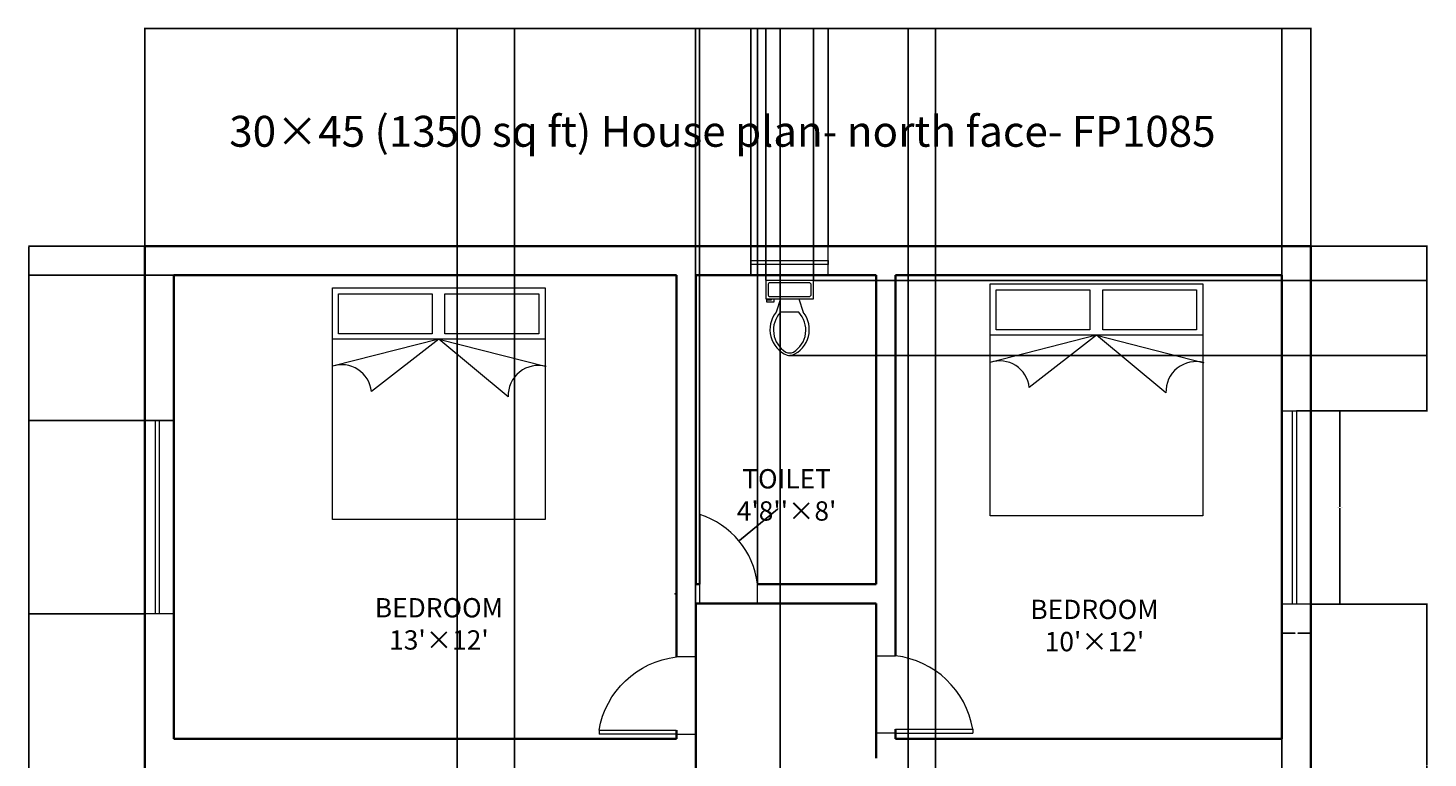
# Model space of a CAD drawing. Units: inches. Extents: x 1108 to 1543, y 442 to 1097.
# Tile 3 of 3: x 1108 to 1543, y 871 to 1097. Entities that reach past the tile are written whole.
import ezdxf

# ---------------------------------------------------------------- set-up
doc = ezdxf.new("R2010")
doc.units = ezdxf.units.IN
for name, color, linetype, lineweight in [('A-ANNO-DIMS', 2, 'Continuous', 18), ('A-ANNO-TEXT', 7, 'Continuous', 25), ('A-AREA-IDEN', 7, 'Continuous', 18), ('A-DOOR', 4, 'Continuous', 18), ('A-FLOR-FIXT', 9, 'Continuous', 18), ('A-FURN', 8, 'Continuous', 18), ('A-GLAZ', 5, 'Continuous', 18), ('A-WALL', 7, 'Continuous', 35)]:
    doc.layers.add(name, color=color, linetype=linetype, lineweight=lineweight)
doc.styles.get("Standard").update_dxf_attribs({"font": 'times.ttf'})
doc.dimstyles.get("Standard").update_dxf_attribs({"dimtxt": 0.18, "dimasz": 0.18, "dimexe": 0.18, "dimexo": 0.0625, "dimgap": 0.09, "dimtad": 0, "dimtih": 1, "dimtoh": 1, "dimdec": 4, "dimzin": 0, "dimdsep": 46, "dimtxsty": 'Standard', "dimcen": 0.09, "dimadec": 0, "dimazin": 0, "dimtfac": 1, "dimtdec": 4, "dimtofl": 0, "dimtmove": 0, "dimatfit": 3, "dimfxl": 1, "dimtolj": 1, "dimtzin": 0, "dimarcsym": 0})

# ---------------------------------------------------------------- blocks, each defined once
blk = doc.blocks.new('d')
for p, q in [((1309.33, 626.48), (1285.33, 626.48)), ((1285.33, 625.28), (1285.33, 626.48)), ((1309.33, 626.48), (1315.33, 626.48)), ((1309.33, 625.28), (1285.33, 625.28)), ((1315.33, 602.48), (1309.33, 602.48))]:
    blk.add_line(p, q)
blk.add_arc((1312.52, 629.86), 27.57, 189.5705, 263.3671)
blk = doc.blocks.new('*U3')
for p, q in [((9.5, -6), (9.5, -2)), ((-10, -8.5), (-8, -8.5)), ((-10, -9.5), (-10, -8.5)), ((-7, -9.5), (-10, -9.5)), ((-8, -8.5), (-8, -8)), ((-7, -8), (-7, -9.5)), ((-4, -8), (-6, -14)), ((4, -8), (6, -14)), ((4, -14), (-4, -14))]:
    blk.add_line(p, q)
blk.add_lwpolyline([(10.5, -8), (10.5, 0), (-10.5, 0), (-10.5, -8)], close=True)
for points in [[(-9.5, -2), (-9.5, -6)], [(8.5, -1), (-8.5, -1)], [(-8.5, -7), (8.5, -7)]]:
    blk.add_lwpolyline(points)
for centre, radius, start, end in [((-8.62, -1.88), 0.884, 81.8699, 188.1301), ((-8.62, -6.12), 0.884, 171.8699, 278.1301), ((8.62, -1.88), 0.884, 351.8699, 98.1301), ((8.62, -6.12), 0.884, 261.8699, 8.1301), ((3.52, -21.58), 12.17, 141.46911, 247.97143), ((4.2, -21.82), 11.33, 136.36773, 238.94682), ((-3.52, -21.58), 12.17, 292.02843, 38.53071), ((-4.2, -21.82), 11.33, 301.05301, 43.63209), ((0, -27.88), 4, 245.73182, 294.26817), ((0, -29), 4, 254.86053, 285.13947)]:
    blk.add_arc(centre, radius, start, end)
blk = doc.blocks.new('BED-DOUBLE-66X72')
for p, q in [((0, 0), (0, 72)), ((0, 72), (66, 72)), ((66, 72), (66, 0)), ((66, 56.1), (0, 56.1)), ((33, 56.1), (0, 47.62)), ((33, 56.1), (12.08, 39.84)), ((33, 56.1), (66, 47.62)), ((54.54, 38.14), (33, 56.1)), ((66, 0), (0, 0))]:
    blk.add_line(p, q)
for points in [[(30.92, 70.13), (30.92, 57.75), (1.83, 57.75), (1.83, 70.13)], [(64.01, 70.13), (64.01, 57.75), (34.92, 57.75), (34.92, 70.13)]]:
    blk.add_lwpolyline(points, close=True)
for centre, radius, start, end in [((2.92, 38.89), 9.21, 5.9499, 108.4921), ((63.85, 38.55), 9.32, 74.4856, 182.5542)]:
    blk.add_arc(centre, radius, start, end)
blk = doc.blocks.new('WIN-60IN')
for p, q in [((-9, -60), (-9, 0)), ((-9, 0), (0, 0)), ((-5.7, -60), (-5.7, 0)), ((0, 0), (-4.5, 0)), ((-4.5, 0), (-4.5, -60)), ((0, 0), (0, -60)), ((0, -60), (-9, -60)), ((-4.5, -60), (-5.7, -60))]:
    blk.add_line(p, q)
blk = doc.blocks.new('*D7')
at = {"layer": 'A-ANNO-DIMS', "color": 0, "lineweight": -2, "transparency": 16777216}
for p, q in [((1506.4, 978.47), (1515.51, 978.47)), ((1515.33, 978.29), (1515.33, 948.65)), ((1515.33, 918.65), (1515.33, 948.29)), ((1506.4, 918.47), (1515.51, 918.47))]:
    blk.add_line(p, q, dxfattribs=at)
at = {"layer": 'A-ANNO-DIMS', "color": 0, "transparency": 16777216}
for points in [[(1515.3, 978.29), (1515.36, 978.29), (1515.33, 978.47)], [(1515.3, 918.65), (1515.36, 918.65), (1515.33, 918.47)]]:
    blk.add_solid(points, dxfattribs=at)
at = {"layer": 'Defpoints', "color": 0, "transparency": 16777216}
for p in [(1506.33, 978.47), (1515.33, 978.47), (1506.33, 918.47)]:
    blk.add_point(p, dxfattribs=at)
at = {"layer": 'A-ANNO-DIMS', "color": 0, "transparency": 16777216, "insert": (1515.33, 948.47), "char_height": 0.18, "attachment_point": 5}
blk.add_mtext('\\A1;WINDOW 60 TYP.', dxfattribs=at)
blk = doc.blocks.new('*D8')
at = {"layer": 'A-ANNO-DIMS', "color": 0, "lineweight": -2, "transparency": 16777216}
for p, q in [((1497.33, 918.41), (1497.33, 909.29)), ((1506.33, 918.41), (1506.33, 909.29)), ((1497.51, 909.47), (1501.38, 909.47)), ((1506.15, 909.47), (1502.29, 909.47))]:
    blk.add_line(p, q, dxfattribs=at)
at = {"layer": 'A-ANNO-DIMS', "color": 0, "transparency": 16777216}
for points in [[(1497.51, 909.5), (1497.51, 909.44), (1497.33, 909.47)], [(1506.15, 909.5), (1506.15, 909.44), (1506.33, 909.47)]]:
    blk.add_solid(points, dxfattribs=at)
at = {"layer": 'Defpoints', "color": 0, "transparency": 16777216}
for p in [(1497.33, 918.47), (1506.33, 918.47), (1506.33, 909.47)]:
    blk.add_point(p, dxfattribs=at)
at = {"layer": 'A-ANNO-DIMS', "color": 0, "transparency": 16777216, "insert": (1501.83, 909.47), "char_height": 0.18, "attachment_point": 5}
blk.add_mtext('\\A1;9 TYP.', dxfattribs=at)
blk = doc.blocks.new('*D15')
at = {"layer": 'A-ANNO-DIMS', "color": 0, "lineweight": -2, "transparency": 16777216}
for p, q in [((1144.33, 1029.74), (1144.33, 1097.43)), ((1144.51, 1097.25), (1325.06, 1097.25)), ((1506.15, 1097.25), (1325.61, 1097.25)), ((1506.33, 1029.74), (1506.33, 1097.43))]:
    blk.add_line(p, q, dxfattribs=at)
at = {"layer": 'A-ANNO-DIMS', "color": 0, "transparency": 16777216}
for points in [[(1144.51, 1097.28), (1144.51, 1097.22), (1144.33, 1097.25)], [(1506.15, 1097.28), (1506.15, 1097.22), (1506.33, 1097.25)]]:
    blk.add_solid(points, dxfattribs=at)
at = {"layer": 'Defpoints', "color": 0, "transparency": 16777216}
for p in [(1506.33, 1097.25), (1144.33, 1029.68), (1506.33, 1029.68)]:
    blk.add_point(p, dxfattribs=at)
at = {"layer": 'A-ANNO-DIMS', "color": 0, "transparency": 16777216, "insert": (1325.33, 1097.25), "char_height": 0.18, "attachment_point": 5}
blk.add_mtext('\\A1;362', dxfattribs=at)
blk = doc.blocks.new('*D16')
at = {"layer": 'A-ANNO-DIMS', "color": 0, "lineweight": -2, "transparency": 16777216}
for p, q in [((1144.27, 1029.68), (1108.2, 1029.68)), ((1108.38, 1029.5), (1108.38, 758.36)), ((1108.38, 486.86), (1108.38, 758)), ((1144.27, 486.68), (1108.2, 486.68))]:
    blk.add_line(p, q, dxfattribs=at)
at = {"layer": 'A-ANNO-DIMS', "color": 0, "transparency": 16777216}
for points in [[(1108.35, 1029.5), (1108.41, 1029.5), (1108.38, 1029.68)], [(1108.35, 486.86), (1108.41, 486.86), (1108.38, 486.68)]]:
    blk.add_solid(points, dxfattribs=at)
at = {"layer": 'Defpoints', "color": 0, "transparency": 16777216}
for p in [(1108.38, 1029.68), (1144.33, 1029.68), (1144.33, 486.68)]:
    blk.add_point(p, dxfattribs=at)
at = {"layer": 'A-ANNO-DIMS', "color": 0, "transparency": 16777216, "insert": (1108.38, 758.18), "char_height": 0.18, "attachment_point": 5}
blk.add_mtext('\\A1;543', dxfattribs=at)
blk = doc.blocks.new('*D17')
at = {"layer": 'A-ANNO-DIMS', "color": 0, "lineweight": -2, "transparency": 16777216}
for p, q in [((1153.27, 1020.68), (1108.2, 1020.68)), ((1108.38, 1020.5), (1108.38, 998.26)), ((1108.38, 975.66), (1108.38, 997.9)), ((1153.27, 975.48), (1108.2, 975.48))]:
    blk.add_line(p, q, dxfattribs=at)
at = {"layer": 'A-ANNO-DIMS', "color": 0, "transparency": 16777216}
for points in [[(1108.35, 1020.5), (1108.41, 1020.5), (1108.38, 1020.68)], [(1108.35, 975.66), (1108.41, 975.66), (1108.38, 975.48)]]:
    blk.add_solid(points, dxfattribs=at)
at = {"layer": 'Defpoints', "color": 0, "transparency": 16777216}
for p in [(1153.33, 1020.68), (1108.38, 975.48), (1153.33, 975.48)]:
    blk.add_point(p, dxfattribs=at)
at = {"layer": 'A-ANNO-DIMS', "color": 0, "transparency": 16777216, "insert": (1108.38, 998.08), "char_height": 0.18, "attachment_point": 5}
blk.add_mtext('\\A1;45.2', dxfattribs=at)
blk = doc.blocks.new('*D18')
at = {"layer": 'A-ANNO-DIMS', "color": 0, "lineweight": -2, "transparency": 16777216}
for p, q in [((1144.27, 915.48), (1108.2, 915.48)), ((1108.38, 915.3), (1108.38, 883.28)), ((1108.38, 850.9), (1108.38, 882.92)), ((1144.27, 850.72), (1108.2, 850.72))]:
    blk.add_line(p, q, dxfattribs=at)
at = {"layer": 'A-ANNO-DIMS', "color": 0, "transparency": 16777216}
for points in [[(1108.35, 915.3), (1108.41, 915.3), (1108.38, 915.48)], [(1108.35, 850.9), (1108.41, 850.9), (1108.38, 850.72)]]:
    blk.add_solid(points, dxfattribs=at)
at = {"layer": 'Defpoints', "color": 0, "transparency": 16777216}
for p in [(1144.33, 915.48), (1108.38, 850.72), (1144.33, 850.72)]:
    blk.add_point(p, dxfattribs=at)
at = {"layer": 'A-ANNO-DIMS', "color": 0, "transparency": 16777216, "insert": (1108.38, 883.1), "char_height": 0.18, "attachment_point": 5}
blk.add_mtext('\\A1;64.76', dxfattribs=at)
blk = doc.blocks.new('*D20')
at = {"layer": 'A-ANNO-DIMS', "color": 0, "lineweight": -2, "transparency": 16777216}
for p, q in [((1506.4, 1029.68), (1542.46, 1029.68)), ((1542.28, 1029.5), (1542.28, 1004.26)), ((1542.28, 978.65), (1542.28, 1003.89)), ((1506.4, 978.47), (1542.46, 978.47))]:
    blk.add_line(p, q, dxfattribs=at)
at = {"layer": 'A-ANNO-DIMS', "color": 0, "transparency": 16777216}
for points in [[(1542.25, 1029.5), (1542.31, 1029.5), (1542.28, 1029.68)], [(1542.25, 978.65), (1542.31, 978.65), (1542.28, 978.47)]]:
    blk.add_solid(points, dxfattribs=at)
at = {"layer": 'Defpoints', "color": 0, "transparency": 16777216}
for p in [(1506.33, 1029.68), (1506.33, 978.47), (1542.28, 978.47)]:
    blk.add_point(p, dxfattribs=at)
at = {"layer": 'A-ANNO-DIMS', "color": 0, "transparency": 16777216, "insert": (1542.28, 1004.08), "char_height": 0.18, "attachment_point": 5}
blk.add_mtext('\\A1;51.21', dxfattribs=at)
blk = doc.blocks.new('*D21')
at = {"layer": 'A-ANNO-DIMS', "color": 0, "lineweight": -2, "transparency": 16777216}
for p, q in [((1506.4, 918.47), (1542.46, 918.47)), ((1542.28, 918.29), (1542.28, 868.51)), ((1542.28, 818.36), (1542.28, 868.14)), ((1506.4, 818.18), (1542.46, 818.18))]:
    blk.add_line(p, q, dxfattribs=at)
at = {"layer": 'A-ANNO-DIMS', "color": 0, "transparency": 16777216}
for points in [[(1542.25, 918.29), (1542.31, 918.29), (1542.28, 918.47)], [(1542.25, 818.36), (1542.31, 818.36), (1542.28, 818.18)]]:
    blk.add_solid(points, dxfattribs=at)
at = {"layer": 'Defpoints', "color": 0, "transparency": 16777216}
for p in [(1506.33, 918.47), (1506.33, 818.18), (1542.28, 818.18)]:
    blk.add_point(p, dxfattribs=at)
at = {"layer": 'A-ANNO-DIMS', "color": 0, "transparency": 16777216, "insert": (1542.28, 868.33), "char_height": 0.18, "attachment_point": 5}
blk.add_mtext('\\A1;100.3', dxfattribs=at)
blk = doc.blocks.new('*D26')
at = {"layer": 'A-ANNO-DIMS', "color": 0, "lineweight": -2, "transparency": 16777216}
for p, q in [((1341.52, 495.74), (1341.52, 1097.43)), ((1341.7, 1097.25), (1361.06, 1097.25)), ((1381.15, 1097.25), (1361.8, 1097.25)), ((1381.33, 495.74), (1381.33, 1097.43))]:
    blk.add_line(p, q, dxfattribs=at)
at = {"layer": 'A-ANNO-DIMS', "color": 0, "transparency": 16777216}
for points in [[(1341.7, 1097.28), (1341.7, 1097.22), (1341.52, 1097.25)], [(1381.15, 1097.28), (1381.15, 1097.22), (1381.33, 1097.25)]]:
    blk.add_solid(points, dxfattribs=at)
at = {"layer": 'Defpoints', "color": 0, "transparency": 16777216}
for p in [(1381.33, 1097.25), (1341.52, 495.68), (1381.33, 495.68)]:
    blk.add_point(p, dxfattribs=at)
at = {"layer": 'A-ANNO-DIMS', "color": 0, "transparency": 16777216, "insert": (1361.43, 1097.25), "char_height": 0.18, "attachment_point": 5}
blk.add_mtext('\\A1;39.81', dxfattribs=at)
blk = doc.blocks.new('*D27')
at = {"layer": 'A-ANNO-DIMS', "color": 0, "lineweight": -2, "transparency": 16777216}
for p, q in [((1332.5, 1029.74), (1332.5, 1097.43)), ((1332.68, 1097.25), (1344.29, 1097.25)), ((1356.32, 1097.25), (1344.72, 1097.25)), ((1356.5, 1029.74), (1356.5, 1097.43))]:
    blk.add_line(p, q, dxfattribs=at)
at = {"layer": 'A-ANNO-DIMS', "color": 0, "transparency": 16777216}
for points in [[(1332.68, 1097.28), (1332.68, 1097.22), (1332.5, 1097.25)], [(1356.32, 1097.28), (1356.32, 1097.22), (1356.5, 1097.25)]]:
    blk.add_solid(points, dxfattribs=at)
at = {"layer": 'Defpoints', "color": 0, "transparency": 16777216}
for p in [(1356.5, 1097.25), (1332.5, 1029.68), (1356.5, 1029.68)]:
    blk.add_point(p, dxfattribs=at)
at = {"layer": 'A-ANNO-DIMS', "color": 0, "transparency": 16777216, "insert": (1344.5, 1097.25), "char_height": 0.18, "attachment_point": 5}
blk.add_mtext('\\A1;24', dxfattribs=at)
blk = doc.blocks.new('*D28')
at = {"layer": 'A-ANNO-DIMS', "color": 0, "lineweight": -2, "transparency": 16777216}
for p, q in [((1315.33, 1020.74), (1315.33, 1097.43)), ((1315.51, 1097.25), (1323.48, 1097.25)), ((1332.32, 1097.25), (1324.35, 1097.25)), ((1332.5, 1020.74), (1332.5, 1097.43))]:
    blk.add_line(p, q, dxfattribs=at)
at = {"layer": 'A-ANNO-DIMS', "color": 0, "transparency": 16777216}
for points in [[(1315.51, 1097.28), (1315.51, 1097.22), (1315.33, 1097.25)], [(1332.32, 1097.28), (1332.32, 1097.22), (1332.5, 1097.25)]]:
    blk.add_solid(points, dxfattribs=at)
at = {"layer": 'Defpoints', "color": 0, "transparency": 16777216}
for p in [(1332.5, 1097.25), (1315.33, 1020.68), (1332.5, 1020.68)]:
    blk.add_point(p, dxfattribs=at)
at = {"layer": 'A-ANNO-DIMS', "color": 0, "transparency": 16777216, "insert": (1323.92, 1097.25), "char_height": 0.18, "attachment_point": 5}
blk.add_mtext('\\A1;17.166', dxfattribs=at)
blk = doc.blocks.new('*D29')
at = {"layer": 'A-ANNO-DIMS', "color": 0, "lineweight": -2, "transparency": 16777216}
for p, q in [((1337.1, 1019.05), (1337.1, 1097.43)), ((1337.28, 1097.25), (1344.15, 1097.25)), ((1351.73, 1097.25), (1344.86, 1097.25)), ((1351.91, 1019.05), (1351.91, 1097.43))]:
    blk.add_line(p, q, dxfattribs=at)
at = {"layer": 'A-ANNO-DIMS', "color": 0, "transparency": 16777216}
for points in [[(1337.28, 1097.28), (1337.28, 1097.22), (1337.1, 1097.25)], [(1351.73, 1097.28), (1351.73, 1097.22), (1351.91, 1097.25)]]:
    blk.add_solid(points, dxfattribs=at)
at = {"layer": 'Defpoints', "color": 0, "transparency": 16777216}
for p in [(1351.91, 1097.25), (1337.1, 1018.98), (1351.91, 1018.98)]:
    blk.add_point(p, dxfattribs=at)
at = {"layer": 'A-ANNO-DIMS', "color": 0, "transparency": 16777216, "insert": (1344.5, 1097.25), "char_height": 0.18, "attachment_point": 5}
blk.add_mtext('\\A1;14.81', dxfattribs=at)
blk = doc.blocks.new('*D30')
at = {"layer": 'A-ANNO-DIMS', "color": 0, "lineweight": -2, "transparency": 16777216}
for p, q in [((1351.97, 1018.98), (1542.46, 1018.98)), ((1542.28, 1018.8), (1542.28, 1007.53)), ((1542.28, 995.89), (1542.28, 1007.17)), ((1344.56, 995.71), (1542.46, 995.71))]:
    blk.add_line(p, q, dxfattribs=at)
at = {"layer": 'A-ANNO-DIMS', "color": 0, "transparency": 16777216}
for points in [[(1542.25, 1018.8), (1542.31, 1018.8), (1542.28, 1018.98)], [(1542.25, 995.89), (1542.31, 995.89), (1542.28, 995.71)]]:
    blk.add_solid(points, dxfattribs=at)
at = {"layer": 'Defpoints', "color": 0, "transparency": 16777216}
for p in [(1351.91, 1018.98), (1542.28, 1018.98), (1344.5, 995.71)]:
    blk.add_point(p, dxfattribs=at)
at = {"layer": 'A-ANNO-DIMS', "color": 0, "transparency": 16777216, "insert": (1542.28, 1007.35), "char_height": 0.18, "attachment_point": 5}
blk.add_mtext('\\A1;23.273', dxfattribs=at)
blk = doc.blocks.new('*D31')
at = {"layer": 'A-ANNO-DIMS', "color": 0, "lineweight": -2, "transparency": 16777216}
for p, q in [((1316.53, 946.34), (1316.53, 1097.43)), ((1316.71, 1097.25), (1325.33, 1097.25)), ((1334.35, 1097.25), (1325.73, 1097.25)), ((1334.53, 924.74), (1334.53, 1097.43))]:
    blk.add_line(p, q, dxfattribs=at)
at = {"layer": 'A-ANNO-DIMS', "color": 0, "transparency": 16777216}
for points in [[(1316.71, 1097.28), (1316.71, 1097.22), (1316.53, 1097.25)], [(1334.35, 1097.28), (1334.35, 1097.22), (1334.53, 1097.25)]]:
    blk.add_solid(points, dxfattribs=at)
at = {"layer": 'Defpoints', "color": 0, "transparency": 16777216}
for p in [(1334.53, 1097.25), (1316.53, 946.28), (1334.53, 924.68)]:
    blk.add_point(p, dxfattribs=at)
at = {"layer": 'A-ANNO-DIMS', "color": 0, "transparency": 16777216, "insert": (1325.53, 1097.25), "char_height": 0.18, "attachment_point": 5}
blk.add_mtext('\\A1;18', dxfattribs=at)
blk = doc.blocks.new('*D49')
at = {"layer": 'A-ANNO-DIMS', "color": 0, "lineweight": -2, "transparency": 16777216}
for p, q in [((1241.29, 854.74), (1241.29, 1097.43)), ((1241.47, 1097.25), (1249.81, 1097.25)), ((1258.89, 1097.25), (1250.55, 1097.25)), ((1259.07, 854.74), (1259.07, 1097.43))]:
    blk.add_line(p, q, dxfattribs=at)
at = {"layer": 'A-ANNO-DIMS', "color": 0, "transparency": 16777216}
for points in [[(1241.47, 1097.28), (1241.47, 1097.22), (1241.29, 1097.25)], [(1258.89, 1097.28), (1258.89, 1097.22), (1259.07, 1097.25)]]:
    blk.add_solid(points, dxfattribs=at)
at = {"layer": 'Defpoints', "color": 0, "transparency": 16777216}
for p in [(1259.07, 1097.25), (1241.29, 854.68), (1259.07, 854.68)]:
    blk.add_point(p, dxfattribs=at)
at = {"layer": 'A-ANNO-DIMS', "color": 0, "transparency": 16777216, "insert": (1250.18, 1097.25), "char_height": 0.18, "attachment_point": 5}
blk.add_mtext('\\A1;17.78', dxfattribs=at)
blk = doc.blocks.new('*D50')
at = {"layer": 'A-ANNO-DIMS', "color": 0, "lineweight": -2, "transparency": 16777216}
for p, q in [((1381.33, 537.14), (1381.33, 1097.43)), ((1381.51, 1097.25), (1385.16, 1097.25)), ((1389.56, 1097.25), (1385.91, 1097.25)), ((1389.74, 537.14), (1389.74, 1097.43))]:
    blk.add_line(p, q, dxfattribs=at)
at = {"layer": 'A-ANNO-DIMS', "color": 0, "transparency": 16777216}
for points in [[(1381.51, 1097.28), (1381.51, 1097.22), (1381.33, 1097.25)], [(1389.56, 1097.28), (1389.56, 1097.22), (1389.74, 1097.25)]]:
    blk.add_solid(points, dxfattribs=at)
at = {"layer": 'Defpoints', "color": 0, "transparency": 16777216}
for p in [(1389.74, 1097.25), (1381.33, 537.08), (1389.74, 537.08)]:
    blk.add_point(p, dxfattribs=at)
at = {"layer": 'A-ANNO-DIMS', "color": 0, "transparency": 16777216, "insert": (1385.54, 1097.25), "char_height": 0.18, "attachment_point": 5}
blk.add_mtext('\\A1;8.404', dxfattribs=at)
blk = doc.blocks.new('*D52')
at = {"layer": 'A-ANNO-DIMS', "color": 0, "lineweight": -2, "transparency": 16777216}
for p, q in [((1315.33, 573.74), (1315.33, 1097.43)), ((1315.51, 1097.25), (1406.07, 1097.25)), ((1497.15, 1097.25), (1406.6, 1097.25)), ((1497.33, 573.74), (1497.33, 1097.43))]:
    blk.add_line(p, q, dxfattribs=at)
at = {"layer": 'A-ANNO-DIMS', "color": 0, "transparency": 16777216}
for points in [[(1315.51, 1097.28), (1315.51, 1097.22), (1315.33, 1097.25)], [(1497.15, 1097.28), (1497.15, 1097.22), (1497.33, 1097.25)]]:
    blk.add_solid(points, dxfattribs=at)
at = {"layer": 'Defpoints', "color": 0, "transparency": 16777216}
for p in [(1497.33, 1097.25), (1315.33, 573.68), (1497.33, 573.68)]:
    blk.add_point(p, dxfattribs=at)
at = {"layer": 'A-ANNO-DIMS', "color": 0, "transparency": 16777216, "insert": (1406.33, 1097.25), "char_height": 0.18, "attachment_point": 5}
blk.add_mtext('\\A1;182', dxfattribs=at)
blk = doc.blocks.new('*D53')
at = {"layer": 'A-ANNO-DIMS', "color": 0, "lineweight": -2, "transparency": 16777216}
for p, q in [((1340.69, 948), (1328.92, 938.24)), ((1340.87, 948), (1340.69, 948)), ((1308.84, 921.68), (1309.02, 921.68)), ((1308.93, 921.59), (1308.93, 921.77))]:
    blk.add_line(p, q, dxfattribs=at)
at = {"layer": 'A-ANNO-DIMS', "color": 0, "transparency": 16777216}
blk.add_solid([(1328.9, 938.27), (1328.94, 938.22), (1328.78, 938.13)], dxfattribs=at)
at = {"layer": 'Defpoints', "color": 0, "transparency": 16777216}
for p in [(1328.78, 938.13), (1308.93, 921.68)]:
    blk.add_point(p, dxfattribs=at)
at = {"layer": 'A-ANNO-DIMS', "color": 0, "transparency": 16777216, "insert": (1341.34, 948), "char_height": 0.18, "attachment_point": 5}
blk.add_mtext('\\A1;R25.78', dxfattribs=at)

msp = doc.modelspace()

# ---------------------------------------------------------------- linework, layer by layer
at = {"layer": 'A-DOOR'}
for p, q in [((1316.5347, 924.6791), (1316.5347, 946.2791)), ((1316.5347, 946.2791), (1316.6347, 946.2791)), ((1316.6347, 946.2791), (1316.6347, 924.6791)), ((1316.6347, 924.6791), (1315.3347, 924.6791)), ((1316.5347, 924.6791), (1316.5347, 918.6791)), ((1316.5347, 924.6791), (1316.6347, 924.6791)), ((1334.5347, 918.6791), (1334.5347, 924.6791)), ((1316.5347, 918.6791), (1334.5347, 918.6791))]:
    msp.add_line(p, q, dxfattribs=at)
msp.add_arc((1308.9321, 921.6791), 25.7777, 6.683214, 72.614123, dxfattribs=at)
at = {"layer": 'A-GLAZ'}
for p, q in [((1356.5008, 1029.6791), (1332.5008, 1029.6791)), ((1332.5008, 1029.6791), (1332.5008, 1020.6791)), ((1356.5008, 1020.6791), (1356.5008, 1029.6791)), ((1332.5008, 1025.1791), (1356.5008, 1025.1791)), ((1356.5008, 1023.9791), (1332.5008, 1023.9791)), ((1356.5008, 1025.1791), (1356.5008, 1023.9791)), ((1332.5008, 1020.6791), (1356.5008, 1020.6791))]:
    msp.add_line(p, q, dxfattribs=at)
at = {"layer": 'A-WALL'}
for p, q in [((1144.3347, 486.6791), (1144.3347, 1029.6791)), ((1144.3347, 1029.6791), (1506.3347, 1029.6791)), ((1506.3347, 486.6791), (1506.3347, 1029.6791)), ((1153.3347, 876.6791), (1153.3347, 1020.6791)), ((1153.3347, 1020.6791), (1309.3347, 1020.6791)), ((1309.3347, 1020.6791), (1309.3347, 902.0778)), ((1315.3347, 1020.6791), (1315.3347, 924.6791)), ((1315.3347, 1020.6791), (1315.3347, 924.6791)), ((1315.3347, 1020.6791), (1371.3347, 1020.6791)), ((1371.3347, 1020.6791), (1371.3347, 924.6791)), ((1377.3347, 1020.6791), (1377.3347, 924.6791)), ((1377.3347, 1020.6791), (1497.3347, 1020.6791)), ((1497.3347, 876.6791), (1497.3347, 1020.6791)), ((1315.3347, 924.6791), (1316.5347, 924.6791)), ((1371.3347, 924.6791), (1334.5347, 924.6791)), ((1377.3347, 918.6791), (1377.3347, 924.6791)), ((1315.3347, 918.6791), (1371.3347, 918.6791)), ((1315.3347, 918.6791), (1315.3347, 828.2882)), ((1371.3347, 918.6791), (1371.3347, 870.6791)), ((1377.3347, 918.6791), (1377.3347, 902.4167)), ((1309.3347, 879.2778), (1309.3347, 876.6791)), ((1377.3347, 879.6167), (1377.3347, 876.6791)), ((1153.3347, 876.6791), (1309.3347, 876.6791)), ((1377.3347, 876.6791), (1497.3347, 876.6791))]:
    msp.add_line(p, q, dxfattribs=at)

# ---------------------------------------------------------------- block references
at = {"layer": 'A-DOOR', "xscale": -1, "rotation": 180}
msp.add_blockref('d', (0, 1504.5569), dxfattribs=at)
at = {"layer": 'A-DOOR', "rotation": 180}
msp.add_blockref('d', (2686.6693, 1504.8958), dxfattribs=at)
at = {"layer": 'A-FLOR-FIXT', "xscale": 0.7052287925630897, "yscale": 0.7052287925630897, "zscale": 0.7052287925630897}
msp.add_blockref('*U3', (1344.5024, 1018.9841), dxfattribs=at)
at = {"layer": 'A-FURN'}
for p in [(1406.7886, 945.9341), (1202.5883, 944.7248)]:
    msp.add_blockref('BED-DOUBLE-66X72', p, dxfattribs=at)
at = {"layer": 'A-GLAZ'}
for p in [(1506.3347, 978.4725), (1153.3347, 975.4836)]:
    msp.add_blockref('WIN-60IN', p, dxfattribs=at)

# ---------------------------------------------------------------- texts
at = {"layer": 'A-ANNO-TEXT', "insert": (1132.9515, 1070.1369), "char_height": 9.6, "attachment_point": 1}
msp.add_mtext_dynamic_manual_height_columns('\\pxqc;30×45 (1350 sq ft) House plan- north face- FP1085', width=381.364536, gutter_width=12.5, heights=[0], dxfattribs=at)
at = {"layer": 'A-AREA-IDEN', "char_height": 6, "attachment_point": 1}
for s, insert in [("\\pxqc;TOILET\\P4'8''×8'", (1209.0015, 960.4092)), ("\\pxqc;BEDROOM \\P13'×12'", (1101.0866, 920.3526)), ("\\pxqc;BEDROOM \\P10'×12'", (1304.5832, 919.839))]:
    msp.add_mtext_dynamic_manual_height_columns(s, width=269.09847, gutter_width=12.5, heights=[0], dxfattribs=dict(at, insert=insert))

# ---------------------------------------------------------------- dimensions: what is measured, and where the dimension line sits
at = {"layer": 'A-ANNO-DIMS'}
for base, p1, p2, override, picture, middle in [((1506.3347, 1097.2479), (1144.3347, 1029.6791), (1506.3347, 1029.6791), {"dimdec": 0, "dimlfac": 1, "dimrnd": 0, "dimzin": 0, "dimdsep": 46, "dimlunit": 2}, '*D15', (1325.3347, 1097.2479)), ((1259.07, 1097.2479), (1241.2895, 854.6808), (1259.07, 854.6808), {"dimdec": 2, "dimlfac": 1, "dimrnd": 0, "dimzin": 0, "dimdsep": 46, "dimlunit": 2}, '*D49', (1250.1797, 1097.2479)), ((1332.5008, 1097.2479), (1315.3347, 1020.6791), (1332.5008, 1020.6791), {"dimdec": 3, "dimlfac": 1, "dimrnd": 0, "dimzin": 0, "dimdsep": 46, "dimlunit": 2}, '*D28', (1323.9177, 1097.2479)), ((1497.3347, 1097.2479), (1315.3347, 573.6791), (1497.3347, 573.6791), {"dimdec": 0, "dimlfac": 1, "dimrnd": 0, "dimzin": 0, "dimdsep": 46, "dimlunit": 2}, '*D52', (1406.3347, 1097.2479)), ((1334.5347, 1097.2479), (1316.5347, 946.2791), (1334.5347, 924.6791), {"dimdec": 0, "dimlfac": 1, "dimrnd": 0, "dimzin": 0, "dimdsep": 46, "dimlunit": 2}, '*D31', (1325.5347, 1097.2479)), ((1356.5008, 1097.2479), (1332.5008, 1029.6791), (1356.5008, 1029.6791), {"dimdec": 0, "dimlfac": 1, "dimrnd": 0, "dimzin": 0, "dimdsep": 46, "dimlunit": 2}, '*D27', (1344.5008, 1097.2479)), ((1351.9073, 1097.2479), (1337.0975, 1018.9841), (1351.9073, 1018.9841), {"dimdec": 2, "dimlfac": 1, "dimrnd": 0, "dimzin": 0, "dimdsep": 46, "dimlunit": 2}, '*D29', (1344.5024, 1097.2479)), ((1381.3347, 1097.2479), (1341.5247, 495.6791), (1381.3347, 495.6791), {"dimdec": 2, "dimlfac": 1, "dimrnd": 0, "dimzin": 0, "dimdsep": 46, "dimlunit": 2}, '*D26', (1361.4297, 1097.2479)), ((1389.7386, 1097.2479), (1381.3347, 537.0791), (1389.7386, 537.0791), {"dimdec": 3, "dimlfac": 1, "dimrnd": 0, "dimzin": 0, "dimdsep": 46, "dimlunit": 2}, '*D50', (1385.5366, 1097.2479))]:
    dim = msp.add_linear_dim(base=base, p1=p1, p2=p2, dimstyle='Standard', override=override, dxfattribs=at)
    dim.commit()
    dim.dimension.update_dxf_attribs({"geometry": picture, "text_midpoint": middle})
for base, p1, p2, override, picture, middle in [((1108.3847, 1029.6791), (1144.3347, 486.6791), (1144.3347, 1029.6791), {"dimdec": 0, "dimlfac": 1, "dimrnd": 0, "dimzin": 0, "dimdsep": 46, "dimlunit": 2}, '*D16', (1108.3847, 758.1791)), ((1542.2847, 978.4725), (1506.3347, 1029.6791), (1506.3347, 978.4725), {"dimdec": 2, "dimlfac": 1, "dimrnd": 0, "dimzin": 0, "dimdsep": 46, "dimlunit": 2}, '*D20', (1542.2847, 1004.0758)), ((1108.3847, 975.4836), (1153.3347, 1020.6791), (1153.3347, 975.4836), {"dimdec": 1, "dimlfac": 1, "dimrnd": 0, "dimzin": 0, "dimdsep": 46, "dimlunit": 2}, '*D17', (1108.3847, 998.0813)), ((1542.28466, 1018.98414), (1344.50239, 995.71161), (1351.90728, 1018.98414), {"dimdec": 3, "dimlfac": 1, "dimrnd": 0, "dimzin": 0, "dimdsep": 46, "dimlunit": 2}, '*D30', (1542.28466, 1007.34787)), ((1542.2847, 818.1791), (1506.3347, 918.4725), (1506.3347, 818.1791), {"dimdec": 1, "dimlfac": 1, "dimrnd": 0, "dimzin": 0, "dimdsep": 46, "dimlunit": 2}, '*D21', (1542.2847, 868.3258)), ((1108.3847, 850.719), (1144.3347, 915.4836), (1144.3347, 850.719), {"dimdec": 2, "dimlfac": 1, "dimrnd": 0, "dimzin": 0, "dimdsep": 46, "dimlunit": 2}, '*D18', (1108.3847, 883.1013))]:
    dim = msp.add_linear_dim(base=base, p1=p1, p2=p2, angle=90, dimstyle='Standard', override=override, dxfattribs=at)
    dim.commit()
    dim.dimension.update_dxf_attribs({"geometry": picture, "text_midpoint": middle})
dim = msp.add_linear_dim(base=(1515.3347, 978.4725), p1=(1506.3347, 918.4725), p2=(1506.3347, 978.4725), angle=90, text='WINDOW <> TYP.', dimstyle='Standard', override={"dimdec": 0, "dimlfac": 1, "dimrnd": 0, "dimzin": 0, "dimdsep": 46, "dimlunit": 2}, dxfattribs=at)
dim.commit()
dim.dimension.update_dxf_attribs({"geometry": '*D7', "text_midpoint": (1515.3347, 948.4725)})
dim = msp.add_radius_dim(center=(1308.9321, 921.6791), mpoint=(1328.7803, 938.1272), dimstyle='Standard', override={"dimdec": 2, "dimlfac": 1, "dimrnd": 0, "dimzin": 0, "dimdsep": 46, "dimlunit": 2}, dxfattribs=at)
dim.commit()
dim.dimension.update_dxf_attribs({"geometry": '*D53', "text_midpoint": (1341.3369, 947.9961), "dimtype": 164})
dim = msp.add_linear_dim(base=(1506.3347, 909.4725), p1=(1497.3347, 918.4725), p2=(1506.3347, 918.4725), text='<> TYP.', dimstyle='Standard', override={"dimdec": 0, "dimlfac": 1, "dimrnd": 0, "dimzin": 0, "dimdsep": 46, "dimlunit": 2}, dxfattribs=at)
dim.commit()
dim.dimension.update_dxf_attribs({"geometry": '*D8', "text_midpoint": (1501.8347, 909.4725)})

doc.saveas('drawing.dxf')
